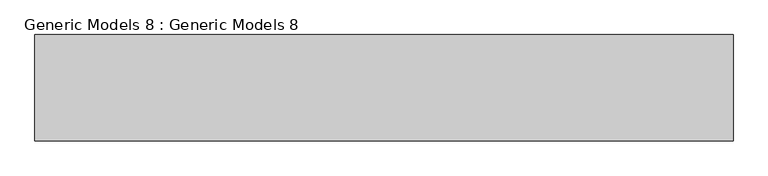
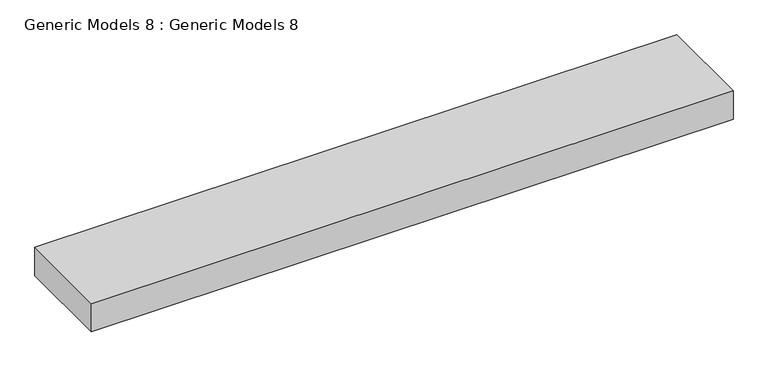
"""IFC4 building model written with IfcOpenShell, lengths in millimetres: proxy geometry, Generic Models 8 : Generic Models 8."""

from ifc_helpers import new_model, si_unit, frame, origin, place, context, project, spatial, polyline, outline, extrude, source, transform, mapped, element, save


def generic_models_8_generic_models_8_4897e18a(model_context):
    return source(origin(), model_context, "Body", "SweptSolid", [
        extrude(outline(polyline([(-7730.0293382, -21294.7893453), (-7730.0293382, -19618.3893453), (3272.4909982, -19618.3893453), (3272.4909982, -21294.7893453), (-7730.0293382, -21294.7893453)])), frame((0.0, 0.0, 15770.5723544), z_axis=(0.0, 0.0, 1.0), x_axis=(1.0, 0.0, 0.0)), (0.0, 0.0, 1.0), 515.6695818),
    ])


if __name__ == "__main__":
    model = new_model("IFC4")
    model_context = context("Model", 3, world=origin())
    ifc_project = project(units=[si_unit("LENGTHUNIT", "METRE", prefix="MILLI")], contexts=[model_context])
    site = spatial("IfcSite", under=ifc_project)
    building = spatial("IfcBuilding", under=site)
    placement = place(None, origin())
    generic_models_8_generic_models_8_shape = generic_models_8_generic_models_8_4897e18a(model_context)
    element("IfcBuildingElementProxy", 1, Name="Generic Models 8 : Generic Models 8", ObjectType="Generic Models 8 : Generic Models 8", at=placement, inside=building, context=model_context, shape_type="MappedRepresentation", body=[
        mapped(generic_models_8_generic_models_8_shape, transform((0.0, 0.0, 0.0), x_axis=(1.0, 0.0, 0.0), y_axis=(0.0, 1.0, 0.0), z_axis=(0.0, 0.0, 1.0))),
    ])
    save(model, "model.ifc")
